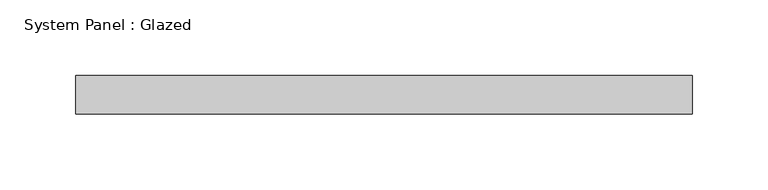
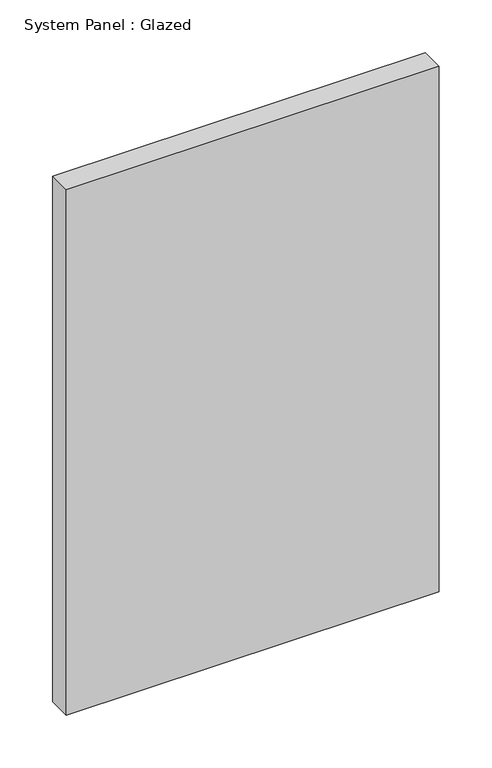
"""IFC4 building model written with IfcOpenShell, lengths in millimetres: plate geometry, System Panel : Glazed."""

from ifc_helpers import new_model, si_unit, origin, origin_with_axes, place, context, project, spatial, polyline, outline, extrude, source, transform, mapped, element, save


def system_panel_glazed_dee09a0e(model_context):
    return source(origin(), model_context, "Body", "SweptSolid", [
        extrude(outline(polyline([(203.2, 19.05), (-203.2, 19.05), (-203.2, 44.45), (203.2, 44.45), (203.2, 19.05)])), origin_with_axes(), (0.0, 0.0, 1.0), 605.4805927),
    ])


if __name__ == "__main__":
    model = new_model("IFC4")
    model_context = context("Model", 3, world=origin())
    ifc_project = project(units=[si_unit("LENGTHUNIT", "METRE", prefix="MILLI")], contexts=[model_context])
    site = spatial("IfcSite", under=ifc_project)
    building = spatial("IfcBuilding", under=site)
    placement = place(None, origin())
    system_panel_glazed_shape = system_panel_glazed_dee09a0e(model_context)
    element("IfcPlate", 1, ObjectType="System Panel : Glazed", at=placement, inside=building, context=model_context, shape_type="MappedRepresentation", body=[
        mapped(system_panel_glazed_shape, transform((0.0, 0.0, 0.0), x_axis=(1.0, 0.0, 0.0), y_axis=(0.0, 1.0, 0.0), z_axis=(0.0, 0.0, 1.0))),
    ])
    save(model, "model.ifc")

# Revit data of these elements
# Type "System Panel : Glazed"
#   Construction Type Id = "GSP4R"
#   Analytic Construction = "1/8 in Pilkington single glazing"
#   Visual Light Transmittance = 0.9
#   Solar Heat Gain Coefficient = 0.86
#   Heat Transfer Coefficient (U) = 1.18115 BTU/(h·ft²·°F)
#   Define Thermal Properties by = 1
# Element 1 (IfcPlate, "System Panel : Glazed")
#   Materials on its faces: "Glass"
# Materials
#   "Glass": class "Glass", colour RGB 0 128 192, transparency 0.75, Description = "Soda Lime Glass", Cost = 0
